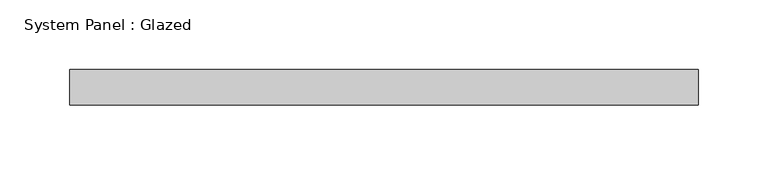
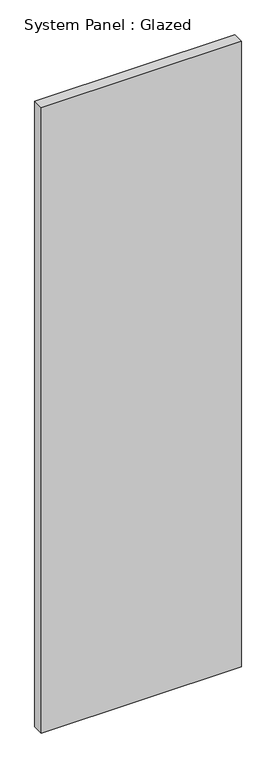
"""IFC4 building model written with IfcOpenShell, lengths in millimetres: plate geometry, System Panel : Glazed."""

from ifc_helpers import new_model, si_unit, origin, origin_with_axes, place, context, project, spatial, polyline, outline, extrude, source, transform, mapped, element, save


def system_panel_glazed_0840b29c(model_context):
    return source(origin(), model_context, "Body", "SweptSolid", [
        extrude(outline(polyline([(225.425, 19.05), (-225.425, 19.05), (-225.425, 44.45), (225.425, 44.45), (225.425, 19.05)])), origin_with_axes(), (0.0, 0.0, 1.0), 1489.3259354),
    ])


if __name__ == "__main__":
    model = new_model("IFC4")
    model_context = context("Model", 3, world=origin())
    ifc_project = project(units=[si_unit("LENGTHUNIT", "METRE", prefix="MILLI")], contexts=[model_context])
    site = spatial("IfcSite", under=ifc_project)
    building = spatial("IfcBuilding", under=site)
    placement = place(None, origin())
    system_panel_glazed_shape = system_panel_glazed_0840b29c(model_context)
    element("IfcPlate", 1, ObjectType="System Panel : Glazed", at=placement, inside=building, context=model_context, shape_type="MappedRepresentation", body=[
        mapped(system_panel_glazed_shape, transform((0.0, 0.0, 0.0), x_axis=(1.0, 0.0, 0.0), y_axis=(0.0, 1.0, 0.0), z_axis=(0.0, 0.0, 1.0))),
    ])
    save(model, "model.ifc")

# Revit data of these elements
# Type "System Panel : Glazed"
#   Construction Type Id = "GSP4R"
#   Analytic Construction = "1/8 in Pilkington single glazing"
#   Visual Light Transmittance = 0.9
#   Solar Heat Gain Coefficient = 0.86
#   Heat Transfer Coefficient (U) = 1.18115 BTU/(h·ft²·°F)
#   Define Thermal Properties by = 1
# Element 1 (IfcPlate, "System Panel : Glazed")
#   Materials on its faces: "Glass"
# Materials
#   "Glass": class "Glass", colour RGB 0 128 192, transparency 0.75, Description = "Soda Lime Glass", Cost = 0
